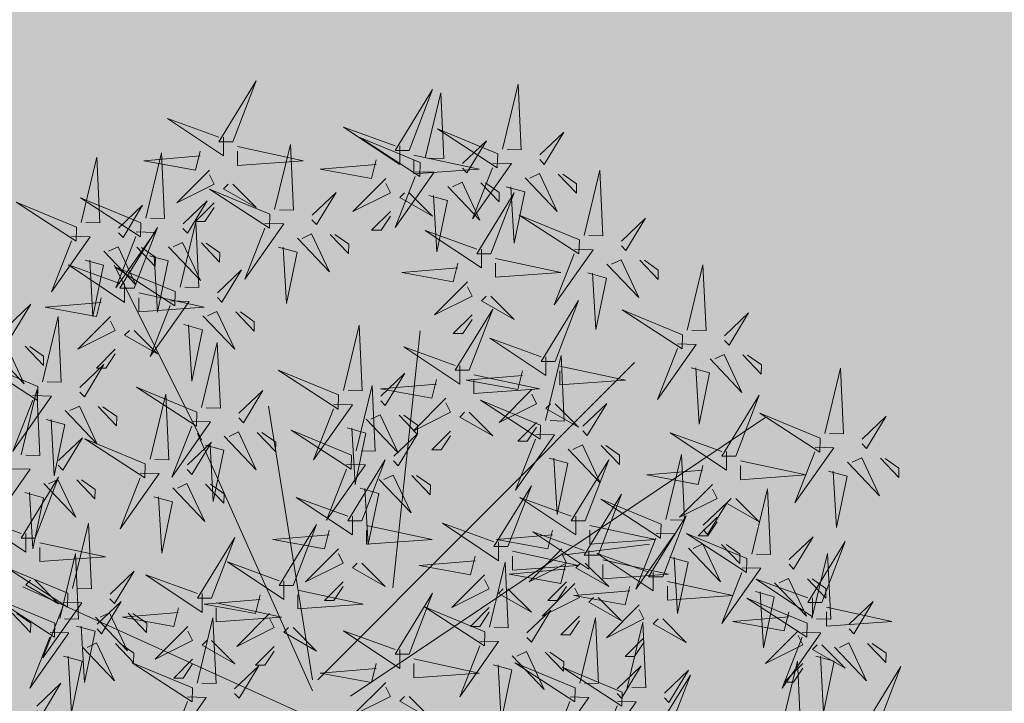
# Model space of a CAD drawing. Units: inches. Extents: x 1704 to 6393, y -157 to 1172.
# Tile 56 of 122: x 1906 to 1931, y 903 to 920. Entities that reach past the tile are written whole.
import ezdxf

# ---------------------------------------------------------------- set-up
doc = ezdxf.new("R2010")
doc.units = ezdxf.units.IN
doc.header["$MEASUREMENT"] = 0
doc.layers.add('A-ANNO-DIMS', color=7, linetype='Continuous', lineweight=13)
doc.layers.add('L-shrub', color=74, linetype='Continuous', lineweight=18)
doc.layers.add('L-HRDS-PATT', color=9, linetype='Continuous', lineweight=13, true_color=0xc5c1ba)
doc.styles.get("Standard").update_dxf_attribs({"font": 'arial.ttf'})
doc.dimstyles.get("Standard").update_dxf_attribs({"dimtxt": 6, "dimasz": 2, "dimexe": 0.18, "dimexo": 0.0625, "dimgap": 0.09, "dimtad": 0, "dimtih": 1, "dimtoh": 1, "dimdec": 1, "dimzin": 0, "dimdsep": 46, "dimlunit": 3, "dimtxsty": 'Standard', "dimblk": 'ARCHTICK', "dimcen": 0.09, "dimadec": 0, "dimazin": 0, "dimtfac": 1, "dimtdec": 1, "dimtofl": 0, "dimtmove": 0, "dimatfit": 3, "dimfxl": 1, "dimtolj": 1, "dimtzin": 0, "dimarcsym": 0})

# ---------------------------------------------------------------- blocks, each defined once
blk = doc.blocks.new('shrub3')
for p, q in [((-5.99, -2.5), (58.67, 140.12)), ((130.91, 52.02), (217.13, 95.08)), ((7.48, -2.5), (134.11, 54.01)), ((12.87, -2.5), (147.58, 19.03)), ((12.87, -5.19), (169.14, -161.27)), ((4.78, -21.34), (142.19, -225.85)), ((58.17, -42.16), (184.8, -55.61)), ((74.33, -125.58), (79.72, -168.64))]:
    blk.add_line(p, q)
for points in [[(85.01, 138.66), (75.77, 138.66), (94.24, 166.33), (85.01, 140.97)], [(157.38, 132.76), (169.66, 162.48), (150.47, 132.94), (157.38, 132.76)], [(116.79, 145.77), (116.56, 136.54), (89.36, 155.7), (114.49, 145.83)], [(40.78, 124.29), (53.06, 154.01), (33.87, 124.47), (40.78, 124.29)], [(175.19, 155.2), (158.65, 139.45), (177.32, 148.22), (175.13, 152.89)], [(55.62, 117.94), (67.9, 147.66), (48.71, 118.11), (55.62, 117.94)], [(186.54, 147.99), (197.78, 136.16), (181.88, 145.8), (184.24, 148.05)], [(45.65, 145.34), (36.2, 136.34), (40.81, 136.22), (45.59, 143.03)], [(82.7, 134.05), (112.71, 122.52), (82.7, 140.97), (82.7, 134.05)], [(123.59, 140.98), (155.69, 133.25), (123.36, 131.75), (123.53, 138.68)], [(152.83, 135.19), (152.6, 125.95), (125.4, 145.11), (150.53, 135.24)], [(235.82, 113.71), (248.1, 143.42), (228.91, 113.88), (235.82, 113.71)], [(36.23, 126.72), (36, 117.49), (8.8, 136.64), (33.93, 126.77)], [(61.92, 134.05), (50.38, 122.52), (59.61, 138.66), (61.92, 136.35)], [(105.09, 139.14), (102.56, 129.96), (77.32, 135.21), (105.04, 136.83)], [(177.09, 138.99), (167.64, 129.99), (172.25, 129.87), (177.04, 136.68)], [(-0.02, 133.17), (11.22, 121.34), (-4.68, 130.97), (-2.32, 133.22)], [(80.39, 131.74), (73.46, 99.46), (71.15, 131.74), (78.08, 131.74)], [(51.07, 120.36), (50.84, 111.13), (23.64, 130.29), (48.77, 120.42)], [(109.47, 129.79), (92.93, 114.04), (111.6, 122.81), (109.41, 127.48)], [(141.13, 128.55), (138.6, 119.38), (113.36, 124.63), (141.08, 126.24)], [(159.63, 130.4), (191.73, 122.67), (159.4, 121.17), (159.57, 128.09)], [(201.04, 101.49), (191.81, 103.79), (196.42, 129.16), (198.73, 101.49)], [(43.03, 121.93), (75.13, 114.2), (42.8, 112.7), (42.97, 119.62)], [(120.82, 122.58), (132.06, 110.75), (116.16, 120.39), (118.52, 122.64)], [(231.27, 116.13), (231.04, 106.9), (203.84, 126.05), (228.97, 116.19)], [(24.53, 120.08), (22, 110.91), (-3.24, 116.16), (24.47, 117.77)], [(145.51, 119.2), (128.97, 103.45), (147.64, 112.22), (145.45, 116.9)], [(207.97, 89.96), (198.73, 89.96), (217.2, 117.63), (207.97, 92.27)], [(39.37, 113.73), (36.84, 104.56), (11.6, 109.81), (39.31, 111.42)], [(57.87, 115.58), (89.97, 107.84), (57.64, 106.34), (57.81, 113.27)], [(111.37, 113.58), (101.92, 104.58), (106.53, 104.46), (111.31, 111.27)], [(156.86, 111.99), (168.1, 100.16), (152.2, 109.8), (154.56, 112.05)], [(191.81, 96.88), (175.65, 113.02), (184.88, 94.57), (189.5, 96.88)], [(237.94, 81.95), (250.22, 111.66), (231.03, 82.12), (237.94, 81.95)], [(28.91, 110.73), (12.37, 94.98), (31.04, 103.75), (28.85, 108.43)], [(119.22, 79.83), (131.5, 109.54), (112.31, 80), (119.22, 79.83)], [(219.57, 109.49), (217.04, 100.32), (191.8, 105.57), (219.52, 107.19)], [(238.07, 111.34), (270.17, 103.61), (237.84, 102.11), (238.01, 109.03)], [(43.75, 104.38), (27.21, 88.63), (45.88, 97.4), (43.69, 102.07)], [(40.26, 103.52), (51.5, 91.69), (35.6, 101.33), (37.96, 103.58)], [(147.41, 102.99), (137.96, 93.99), (142.57, 93.88), (147.36, 100.68)], [(175.65, 94.57), (166.41, 103.79), (166.41, 99.18), (173.34, 94.57)], [(55.1, 97.17), (66.34, 85.34), (50.44, 94.98), (52.8, 97.23)], [(223.95, 100.15), (207.41, 84.4), (226.08, 93.17), (223.89, 97.84)], [(30.81, 94.52), (21.36, 85.52), (25.97, 85.41), (30.75, 92.21)], [(114.67, 82.25), (114.44, 73.02), (87.24, 92.18), (112.37, 82.31)], [(204.02, 65.01), (216.3, 94.72), (197.11, 65.18), (204.02, 65.01)], [(205.66, 85.35), (235.67, 73.82), (205.66, 92.27), (205.66, 85.35)], [(233.39, 84.37), (233.16, 75.14), (205.96, 94.29), (231.09, 84.43)], [(235.3, 92.94), (246.54, 81.11), (230.64, 90.74), (233, 92.99)], [(45.65, 88.17), (36.2, 79.17), (40.81, 79.05), (45.59, 85.86)], [(48.4, 63.38), (39.16, 65.68), (43.78, 91.04), (46.09, 63.38)], [(184.88, 85.35), (173.34, 73.82), (182.57, 89.96), (184.88, 87.65)], [(8.98, 56.54), (21.26, 86.25), (2.07, 56.71), (8.98, 56.54)], [(144.66, 54.42), (156.94, 84.13), (137.75, 54.59), (144.66, 54.42)], [(203.35, 83.04), (196.42, 50.76), (194.11, 83.04), (201.04, 83.04)], [(225.85, 83.93), (216.4, 74.93), (221.01, 74.82), (225.8, 81.63)], [(55.33, 51.85), (46.09, 51.85), (64.56, 79.52), (55.33, 54.15)], [(221.69, 77.73), (219.16, 68.56), (193.92, 73.81), (221.64, 75.43)], [(240.19, 79.58), (272.29, 71.85), (239.96, 70.35), (240.13, 77.27)], [(273.12, 52.79), (263.89, 55.09), (268.5, 80.46), (270.81, 52.79)], [(39.16, 58.76), (23, 74.9), (32.24, 56.46), (36.86, 58.76)], [(102.97, 75.62), (100.44, 66.44), (75.2, 71.69), (102.92, 73.31)], [(121.47, 77.46), (153.57, 69.73), (121.24, 68.23), (121.41, 75.15)], [(199.47, 67.43), (199.24, 58.2), (172.04, 77.35), (197.17, 67.49)], [(4.43, 58.96), (4.2, 49.73), (-23, 68.88), (2.13, 59.02)], [(226.07, 68.39), (209.53, 52.64), (228.2, 61.41), (226.01, 66.08)], [(280.05, 41.26), (270.81, 41.26), (289.28, 68.93), (280.05, 43.57)], [(23, 56.46), (13.77, 65.68), (13.77, 61.07), (20.7, 56.46)], [(107.35, 66.27), (90.81, 50.52), (109.48, 59.29), (107.29, 63.96)], [(140.11, 56.84), (139.88, 47.61), (112.68, 66.77), (137.81, 56.9)], [(263.89, 48.18), (247.73, 64.32), (256.96, 45.87), (261.58, 48.18)], [(118.7, 59.06), (129.94, 47.23), (114.04, 56.86), (116.4, 59.12)], [(187.77, 60.79), (185.24, 51.62), (160, 56.87), (187.72, 58.49)], [(206.27, 62.64), (238.37, 54.91), (206.04, 53.41), (206.21, 60.33)], [(237.42, 61.17), (248.66, 49.35), (232.76, 58.98), (235.12, 61.23)], [(11.23, 54.17), (43.33, 46.44), (11, 44.94), (11.17, 51.86)], [(53.02, 47.24), (83.03, 35.71), (53.02, 54.15), (53.02, 47.24)], [(247.73, 45.87), (238.49, 55.09), (238.49, 50.48), (245.42, 45.87)], [(32.24, 47.24), (20.7, 35.71), (29.93, 51.85), (32.24, 49.54)], [(54.76, 23.15), (45.52, 25.45), (50.14, 50.81), (52.45, 23.15)], [(109.25, 50.06), (99.8, 41.06), (104.41, 40.94), (109.19, 47.75)], [(128.41, 50.21), (125.88, 41.03), (100.64, 46.28), (128.36, 47.9)], [(146.91, 52.05), (179.01, 44.32), (146.68, 42.82), (146.85, 49.75)], [(192.15, 51.45), (175.61, 35.7), (194.28, 44.47), (192.09, 49.14)], [(227.97, 52.17), (218.52, 43.17), (223.13, 43.06), (227.92, 49.87)], [(50.71, 44.93), (43.78, 12.65), (41.47, 44.93), (48.4, 44.93)], [(203.5, 44.24), (214.74, 32.41), (198.84, 42.04), (201.2, 44.29)], [(242.18, 18.42), (254.46, 48.14), (235.27, 18.6), (242.18, 18.42)], [(61.69, 11.62), (52.45, 11.62), (70.92, 39.29), (61.69, 13.92)], [(132.79, 40.86), (116.25, 25.11), (134.92, 33.88), (132.73, 38.55)], [(256.96, 36.65), (245.42, 25.12), (254.65, 41.26), (256.96, 38.95)], [(277.74, 36.65), (307.75, 25.12), (277.74, 43.57), (277.74, 36.65)], [(8.46, 35.77), (19.7, 23.94), (3.8, 33.57), (6.16, 35.82)], [(45.52, 18.53), (29.36, 34.67), (38.6, 16.23), (43.22, 18.53)], [(194.05, 35.23), (184.6, 26.23), (189.21, 26.12), (194, 32.93)], [(275.43, 34.34), (268.5, 2.06), (266.19, 34.34), (273.12, 34.34)], [(144.14, 33.65), (155.38, 21.82), (139.48, 31.46), (141.84, 33.71)], [(237.63, 20.85), (237.4, 11.62), (210.2, 30.77), (235.33, 20.91)], [(29.36, 16.23), (20.13, 25.45), (20.13, 20.84), (27.06, 16.23)], [(134.69, 24.65), (125.24, 15.65), (129.85, 15.53), (134.63, 22.34)], [(86.56, -10.73), (77.32, -8.43), (81.94, 16.94), (84.25, -10.73)], [(244.43, 16.06), (276.53, 8.33), (244.2, 6.83), (244.37, 13.75)], [(38.6, 7), (27.06, -4.52), (36.29, 11.62), (38.6, 9.31)], [(59.38, 7), (89.39, -4.52), (59.38, 13.92), (59.38, 7)], [(153.14, -15.45), (165.42, 14.26), (146.23, -15.28), (153.14, -15.45)], [(225.93, 14.21), (223.4, 5.04), (198.16, 10.29), (225.88, 11.9)], [(93.49, -22.26), (84.25, -22.26), (102.72, 5.41), (93.49, -19.96)], [(123.46, -21.81), (135.74, 7.91), (116.55, -21.63), (123.46, -21.81)], [(230.31, 4.87), (213.77, -10.89), (232.44, -2.12), (230.25, 2.56)], [(57.07, 4.7), (50.14, -27.58), (47.83, 4.7), (54.76, 4.7)], [(77.32, -15.34), (61.16, 0.8), (70.4, -17.65), (75.02, -15.34)], [(148.59, -13.03), (148.36, -22.26), (121.16, -3.11), (146.29, -12.97)], [(241.66, -2.35), (252.9, -14.18), (237, -4.54), (239.36, -2.29)], [(20.84, -34.02), (11.6, -31.72), (16.22, -6.36), (18.53, -34.02)], [(61.16, -17.65), (51.93, -8.43), (51.93, -13.04), (58.86, -17.65)], [(118.91, -19.38), (118.68, -28.61), (91.48, -9.46), (116.61, -19.33)], [(268.88, -34.02), (259.65, -31.72), (264.26, -6.36), (266.57, -34.02)], [(232.21, -11.35), (222.76, -20.35), (227.37, -20.46), (232.16, -13.66)], [(27.76, -45.55), (18.53, -45.55), (37, -17.88), (27.76, -43.25)], [(155.39, -17.82), (187.49, -25.55), (155.16, -27.05), (155.33, -20.13)], [(275.81, -45.55), (266.57, -45.55), (285.04, -17.88), (275.81, -43.25)], [(11.6, -38.64), (-4.56, -22.5), (4.68, -40.94), (9.3, -38.64)], [(70.4, -26.87), (58.86, -38.4), (68.09, -22.26), (70.4, -24.57)], [(91.18, -26.87), (121.19, -38.4), (91.18, -19.96), (91.18, -26.87)], [(136.89, -19.67), (134.36, -28.84), (109.12, -23.59), (136.84, -21.97)], [(125.71, -24.17), (157.81, -31.9), (125.48, -33.4), (125.65, -26.48)], [(259.65, -38.64), (243.49, -22.5), (252.72, -40.94), (257.34, -38.64)], [(107.21, -26.02), (104.68, -35.19), (79.44, -29.94), (107.16, -28.33)], [(141.27, -29.01), (124.73, -44.76), (143.4, -35.99), (141.21, -31.32)], [(267.62, -55.68), (279.9, -25.97), (260.71, -55.51), (267.62, -55.68)], [(88.87, -29.18), (81.94, -61.46), (79.63, -29.18), (86.56, -29.18)], [(243.49, -40.94), (234.25, -31.72), (234.25, -36.33), (241.18, -40.94)], [(111.59, -35.37), (95.05, -51.12), (113.72, -42.35), (111.53, -37.67)], [(152.62, -36.23), (163.86, -48.05), (147.96, -38.42), (150.32, -36.17)], [(160.76, -63.67), (151.53, -61.36), (156.14, -36), (158.45, -63.67)], [(25.46, -50.16), (55.47, -61.69), (25.46, -43.25), (25.46, -50.16)], [(122.94, -42.58), (134.18, -54.41), (118.28, -44.77), (120.64, -42.52)], [(263.07, -53.26), (262.84, -62.49), (235.64, -43.34), (260.77, -53.2)], [(273.5, -50.16), (303.51, -61.69), (273.5, -43.25), (273.5, -50.16)], [(4.68, -50.16), (-6.86, -61.69), (2.37, -45.55), (4.68, -47.86)], [(143.17, -45.23), (133.72, -54.23), (138.33, -54.34), (143.12, -47.53)], [(167.69, -75.2), (158.45, -75.2), (176.92, -47.53), (167.69, -72.89)], [(218, -74.25), (208.77, -71.95), (213.38, -46.59), (215.69, -74.25)], [(252.72, -50.16), (241.18, -61.69), (250.41, -45.55), (252.72, -47.86)], [(23.15, -52.47), (16.22, -84.75), (13.91, -52.47), (20.84, -52.47)], [(113.49, -51.58), (104.04, -60.58), (108.65, -60.69), (113.43, -53.89)], [(151.53, -68.28), (135.37, -52.14), (144.6, -70.59), (149.22, -68.28)], [(271.19, -52.47), (264.26, -84.75), (261.95, -52.47), (268.88, -52.47)], [(36.54, -87.45), (48.82, -57.73), (29.63, -87.27), (36.54, -87.45)], [(73.84, -82.72), (64.6, -80.42), (69.22, -55.06), (71.53, -82.72)], [(224.93, -85.78), (215.69, -85.78), (234.16, -58.11), (224.93, -83.48)], [(269.87, -58.05), (301.97, -65.78), (269.64, -67.28), (269.81, -60.36)], [(135.37, -70.59), (126.13, -61.36), (126.13, -65.97), (133.06, -70.59)], [(208.77, -78.87), (192.61, -62.73), (201.84, -81.17), (206.46, -78.87)], [(251.37, -59.9), (248.84, -69.07), (223.6, -63.82), (251.32, -62.2)], [(80.77, -94.25), (71.53, -94.25), (90, -66.58), (80.77, -91.95)], [(271.86, -93.8), (284.14, -64.08), (264.95, -93.62), (271.86, -93.8)], [(64.6, -87.34), (48.44, -71.2), (57.68, -89.64), (62.3, -87.34)], [(192.61, -81.17), (183.37, -71.95), (183.37, -76.56), (190.3, -81.17)], [(255.75, -69.24), (239.21, -85), (257.88, -76.23), (255.7, -71.55)], [(31.99, -85.02), (31.76, -94.25), (4.56, -75.1), (29.69, -84.96)], [(144.6, -79.81), (133.06, -91.34), (142.29, -75.2), (144.6, -77.5)], [(165.38, -79.81), (195.39, -91.34), (165.38, -72.89), (165.38, -79.81)], [(267.1, -76.46), (278.34, -88.28), (262.44, -78.65), (264.8, -76.4)], [(48.44, -89.64), (39.21, -80.42), (39.21, -85.03), (46.14, -89.64)], [(163.07, -82.11), (156.14, -114.39), (153.83, -82.11), (160.76, -82.11)], [(165, -106.02), (155.77, -103.71), (160.38, -78.35), (162.69, -106.02)], [(267.31, -91.37), (267.08, -100.61), (239.88, -81.45), (265.01, -91.32)], [(138.3, -114.97), (150.58, -85.26), (131.39, -114.8), (138.3, -114.97)], [(201.84, -90.4), (190.3, -101.92), (199.53, -85.78), (201.84, -88.09)], [(222.62, -90.4), (252.63, -101.92), (222.62, -83.48), (222.62, -90.4)], [(257.65, -85.46), (248.2, -94.46), (252.81, -94.57), (257.6, -87.76)], [(20.29, -91.66), (17.76, -100.83), (-7.48, -95.58), (20.23, -93.97)], [(38.79, -89.81), (70.89, -97.54), (38.56, -99.04), (38.73, -92.12)], [(78.46, -98.86), (108.47, -110.39), (78.46, -91.95), (78.46, -98.86)], [(171.93, -117.54), (162.69, -117.54), (181.16, -89.88), (171.93, -115.24)], [(57.68, -98.86), (46.14, -110.39), (55.37, -94.25), (57.68, -96.56)], [(86.56, -120.84), (77.32, -118.53), (81.94, -93.17), (84.25, -120.84)], [(155.77, -110.63), (139.61, -94.49), (148.84, -112.93), (153.46, -110.63)], [(220.31, -92.7), (213.38, -124.98), (211.07, -92.7), (218, -92.7)], [(274.11, -96.16), (306.21, -103.89), (273.88, -105.4), (274.05, -98.47)], [(24.67, -101), (8.13, -116.76), (26.8, -107.99), (24.61, -103.31)], [(69.6, -127.19), (60.36, -124.88), (64.98, -99.52), (67.29, -127.19)], [(76.15, -101.17), (69.22, -133.45), (66.91, -101.17), (73.84, -101.17)], [(255.61, -98.01), (253.08, -107.18), (227.84, -101.93), (255.56, -100.32)], [(8.98, -131.91), (21.26, -102.2), (2.07, -131.74), (8.98, -131.91)], [(93.49, -132.37), (84.25, -132.37), (102.72, -104.7), (93.49, -130.06)], [(133.75, -112.55), (133.52, -121.78), (106.32, -102.62), (131.45, -112.49)], [(139.61, -112.93), (130.37, -103.71), (130.37, -108.32), (137.3, -112.93)], [(229.46, -134.03), (241.74, -104.31), (222.55, -133.86), (229.46, -134.03)], [(36.02, -108.22), (47.26, -120.04), (31.36, -110.41), (33.72, -108.16)], [(77.32, -125.45), (61.16, -109.31), (70.4, -127.75), (75.02, -125.45)], [(76.53, -138.72), (67.29, -138.72), (85.76, -111.05), (76.53, -136.41)], [(259.99, -107.36), (243.45, -123.11), (262.12, -114.34), (259.94, -109.66)], [(60.36, -131.8), (44.2, -115.66), (53.44, -134.11), (58.06, -131.8)], [(169.62, -122.16), (199.63, -133.69), (169.62, -115.24), (169.62, -122.16)], [(271.34, -114.57), (282.58, -126.4), (266.68, -116.76), (269.04, -114.51)], [(4.43, -129.49), (4.2, -138.72), (-23, -119.56), (2.13, -129.43)], [(26.57, -117.22), (17.12, -126.22), (21.73, -126.33), (26.51, -119.53)], [(61.16, -127.75), (51.93, -118.53), (51.93, -123.14), (58.86, -127.75)], [(122.05, -119.18), (119.52, -128.36), (94.28, -123.11), (122, -121.49)], [(148.84, -122.16), (137.3, -133.69), (146.53, -117.54), (148.84, -119.85)], [(140.55, -117.34), (172.65, -125.07), (140.32, -126.57), (140.49, -119.65)], [(6.86, -155.2), (19.14, -125.49), (-0.05, -155.03), (6.86, -155.2)], [(44.2, -134.11), (34.97, -124.88), (34.97, -129.5), (41.9, -134.11)], [(167.31, -124.46), (160.38, -156.74), (158.07, -124.46), (165, -124.46)], [(224.91, -131.61), (224.68, -140.84), (197.48, -121.68), (222.61, -131.55)], [(261.89, -123.57), (252.44, -132.57), (257.05, -132.69), (261.84, -125.88)], [(91.18, -136.98), (121.19, -148.51), (91.18, -130.06), (91.18, -136.98)], [(126.43, -128.53), (109.89, -144.28), (128.56, -135.51), (126.37, -130.84)], [(11.23, -134.28), (43.33, -142.01), (11, -143.51), (11.17, -136.58)], [(59, -158.95), (49.76, -156.64), (54.38, -131.28), (56.69, -158.95)], [(70.4, -136.98), (58.86, -148.51), (68.09, -132.37), (70.4, -134.67)], [(137.78, -135.74), (149.02, -147.57), (133.12, -137.94), (135.48, -135.69)], [(53.44, -143.33), (41.9, -154.86), (51.13, -138.72), (53.44, -141.02)], [(74.22, -143.33), (104.23, -154.86), (74.22, -136.41), (74.22, -143.33)], [(88.87, -139.28), (81.94, -171.56), (79.63, -139.28), (86.56, -139.28)], [(213.21, -138.24), (210.68, -147.41), (185.44, -142.16), (213.16, -140.55)], [(231.71, -136.39), (263.81, -144.13), (231.48, -145.63), (231.65, -138.7)], [(2.31, -152.78), (2.08, -162.01), (-25.12, -142.86), (0.01, -152.72)], [(65.93, -170.48), (56.69, -170.48), (75.16, -142.81), (65.93, -168.17)], [(89.54, -174.26), (101.82, -144.54), (82.63, -174.09), (89.54, -174.26)], [(128.33, -144.74), (118.88, -153.74), (123.49, -153.86), (128.27, -147.05)], [(49.76, -163.56), (33.6, -147.42), (42.84, -165.87), (47.46, -163.56)], [(71.91, -145.64), (64.98, -177.92), (62.67, -145.64), (69.6, -145.64)], [(217.59, -147.59), (201.05, -163.34), (219.72, -154.57), (217.53, -149.9)], [(8.46, -152.68), (19.7, -164.51), (3.8, -154.87), (6.16, -152.62)], [(182.82, -184.85), (195.1, -155.13), (175.91, -184.67), (182.82, -184.85)], [(228.94, -154.8), (240.18, -166.63), (224.28, -156.99), (226.64, -154.74)], [(9.11, -157.57), (41.21, -165.3), (8.88, -166.8), (9.05, -159.88)], [(33.6, -165.87), (24.37, -156.64), (24.37, -161.26), (31.3, -165.87)], [(84.99, -171.84), (84.76, -181.07), (57.56, -161.91), (82.69, -171.78)], [(219.49, -163.8), (210.04, -172.8), (214.65, -172.92), (219.44, -166.11)], [(63.62, -175.09), (93.63, -186.62), (63.62, -168.17), (63.62, -175.09)], [(118.36, -194.95), (109.13, -192.64), (113.74, -167.28), (116.05, -194.95)], [(-14.82, -177.21), (15.19, -188.74), (-14.82, -170.29), (-14.82, -177.21)], [(42.84, -175.09), (31.3, -186.62), (40.53, -170.48), (42.84, -172.79)], [(178.27, -182.42), (178.04, -191.65), (150.84, -172.5), (175.97, -182.36)], [(6.34, -175.97), (17.58, -187.8), (1.68, -178.17), (4.04, -175.92)], [(73.29, -178.47), (70.76, -187.64), (45.52, -182.39), (73.23, -180.78)], [(61.31, -177.4), (54.38, -209.68), (52.07, -177.4), (59, -177.4)], [(91.79, -176.62), (123.89, -184.36), (91.56, -185.86), (91.73, -178.93)], [(125.29, -206.48), (116.05, -206.48), (134.52, -178.81), (125.29, -204.17)], [(109.13, -199.56), (92.96, -183.42), (102.2, -201.86), (106.82, -199.56)], [(77.67, -187.82), (61.13, -203.57), (79.8, -194.8), (77.61, -190.13)], [(72.58, -216.61), (84.86, -186.89), (65.67, -216.43), (72.58, -216.61)], [(166.57, -189.06), (164.04, -198.23), (138.8, -192.98), (166.52, -191.37)], [(185.07, -187.21), (217.17, -194.94), (184.84, -196.44), (185.01, -189.52)], [(92.96, -201.86), (83.73, -192.64), (83.73, -197.25), (90.66, -201.86)], [(89.02, -195.03), (100.26, -206.86), (84.36, -197.22), (86.72, -194.97)], [(170.95, -198.4), (154.41, -214.16), (173.08, -205.39), (170.89, -200.71)], [(68.03, -214.18), (67.8, -223.42), (40.6, -204.26), (65.73, -214.13)], [(79.57, -204.03), (70.12, -213.03), (74.73, -213.15), (79.51, -206.34)], [(102.2, -211.09), (90.66, -222.62), (99.89, -206.48), (102.2, -208.78)], [(122.98, -211.09), (152.99, -222.62), (122.98, -204.17), (122.98, -211.09)], [(182.3, -205.62), (193.54, -217.44), (177.64, -207.81), (180, -205.56)], [(46.28, -237.29), (37.04, -234.99), (41.66, -209.63), (43.97, -237.29)], [(120.67, -213.39), (113.74, -245.67), (111.43, -213.39), (118.36, -213.39)], [(40.78, -246.25), (53.06, -216.54), (33.87, -246.08), (40.78, -246.25)], [(172.85, -214.62), (163.4, -223.62), (168.01, -223.73), (172.8, -216.93)], [(56.33, -220.82), (53.8, -229.99), (28.56, -224.74), (56.27, -223.13)], [(53.21, -248.82), (43.97, -248.82), (62.44, -221.15), (53.21, -246.52)], [(74.83, -218.97), (106.93, -226.7), (74.6, -228.2), (74.77, -221.28)], [(131.94, -252.6), (144.22, -222.89), (125.03, -252.43), (131.94, -252.6)], [(37.04, -241.91), (20.88, -225.77), (30.12, -244.21), (34.74, -241.91)], [(60.71, -230.17), (44.17, -245.92), (62.84, -237.15), (60.65, -232.47)], [(-9.97, -233.79), (22.13, -241.53), (-10.2, -243.03), (-10.03, -236.1)], [(36.23, -243.83), (36, -253.06), (8.8, -233.9), (33.93, -243.77)], [(20.88, -244.21), (11.65, -234.99), (11.65, -239.6), (18.58, -244.21)], [(72.06, -237.38), (83.3, -249.21), (67.4, -239.57), (69.76, -237.32)], [(127.39, -250.18), (127.16, -259.41), (99.96, -240.26), (125.09, -250.12)], [(50.9, -253.43), (80.91, -264.96), (50.9, -246.52), (50.9, -253.43)], [(62.61, -246.38), (53.16, -255.38), (57.77, -255.49), (62.55, -248.69)], [(24.53, -250.46), (22, -259.64), (-3.24, -254.39), (24.47, -252.77)], [(30.12, -253.43), (18.58, -264.96), (27.81, -248.82), (30.12, -251.13)], [(43.03, -248.62), (75.13, -256.35), (42.8, -257.85), (42.97, -250.92)], [(48.59, -255.74), (41.66, -288.02), (39.35, -255.74), (46.28, -255.74)], [(115.69, -256.81), (113.16, -265.99), (87.92, -260.74), (115.64, -259.12)], [(134.19, -254.97), (166.29, -262.7), (133.96, -264.2), (134.13, -257.28)], [(28.91, -259.81), (12.37, -275.56), (31.04, -266.79), (28.85, -262.12)], [(120.07, -266.16), (103.53, -281.91), (122.2, -273.14), (120.01, -268.47)], [(40.26, -267.02), (51.5, -278.85), (35.6, -269.21), (37.96, -266.96)], [(-10.58, -280.96), (19.43, -292.49), (-10.58, -274.04), (-10.58, -280.96)], [(30.81, -276.02), (21.36, -285.02), (25.97, -285.14), (30.75, -278.33)], [(131.42, -273.37), (142.66, -285.2), (126.76, -275.57), (129.12, -273.32)], [(121.97, -282.37), (112.52, -291.38), (117.13, -291.49), (121.91, -284.68)]]:
    blk.add_lwpolyline(points)
blk = doc.blocks.new('_ArchTick')
at = {"color": 0, "linetype": 'ByBlock', "const_width": 0.15}
blk.add_lwpolyline([(-0.5, -0.5), (0.5, 0.5)], dxfattribs=at)
blk = doc.blocks.new('*D94')
at = {"layer": 'A-ANNO-DIMS', "color": 0, "lineweight": -2, "transparency": 16777216}
for p, q in [((1898.349, 895.275), (1898.349, 1105.287)), ((1898.349, 1105.107), (1979.39, 1105.107)), ((2073.349, 1105.107), (1992.307, 1105.107)), ((2073.349, 895.275), (2073.349, 1105.287))]:
    blk.add_line(p, q, dxfattribs=at)
at = {"layer": 'Defpoints', "color": 0, "lineweight": -3, "transparency": 16777216}
for p in [(2073.349, 1105.107), (1898.349, 895.213), (2073.349, 895.213)]:
    blk.add_point(p, dxfattribs=at)
at = {"layer": 'A-ANNO-DIMS', "color": 0, "lineweight": -2, "transparency": 16777216, "xscale": 2, "yscale": 2, "zscale": 2, "rotation": 180}
blk.add_blockref('_ArchTick', (1898.349, 1105.107), dxfattribs=at)
at = {"layer": 'A-ANNO-DIMS', "color": 0, "lineweight": -2, "transparency": 16777216, "xscale": 2, "yscale": 2, "zscale": 2}
blk.add_blockref('_ArchTick', (2073.349, 1105.107), dxfattribs=at)
at = {"layer": 'A-ANNO-DIMS', "color": 0, "transparency": 16777216, "insert": (1985.849, 1105.107), "char_height": 6, "attachment_point": 5}
blk.add_mtext('\\A1;175', dxfattribs=at)

msp = doc.modelspace()

# ---------------------------------------------------------------- hatches: boundary and pattern name
at = {"layer": 'L-HRDS-PATT', "transparency": 33554643}
h = msp.add_hatch(color=256, dxfattribs=at)
h.dxf.hatch_style = 1
h.paths.add_polyline_path([(2065.589, 1033.213), (1898.349, 1033.213), (1898.349, 895.213), (2065.589, 895.213)])

# ---------------------------------------------------------------- block references
at = {"layer": 'L-shrub', "xscale": 0.0510581485411622, "yscale": 0.0510581485411622, "zscale": 0.0510581485411622, "rotation": 89.99999999999996}
msp.add_blockref('shrub3', (1913.464, 903.144), dxfattribs=at)

# ---------------------------------------------------------------- dimensions: what is measured, and where the dimension line sits
at = {"layer": 'A-ANNO-DIMS'}
dim = msp.add_linear_dim(base=(2073.349, 1105.107), p1=(1898.349, 895.213), p2=(2073.349, 895.213), dimstyle='Standard', override={"dimdec": 0, "dimlfac": 1, "dimrnd": 0, "dimzin": 0, "dimdsep": 46, "dimlunit": 2}, dxfattribs=at)
dim.commit()
dim.dimension.update_dxf_attribs({"geometry": '*D94', "text_midpoint": (1985.849, 1105.107)})

doc.saveas('drawing.dxf')
